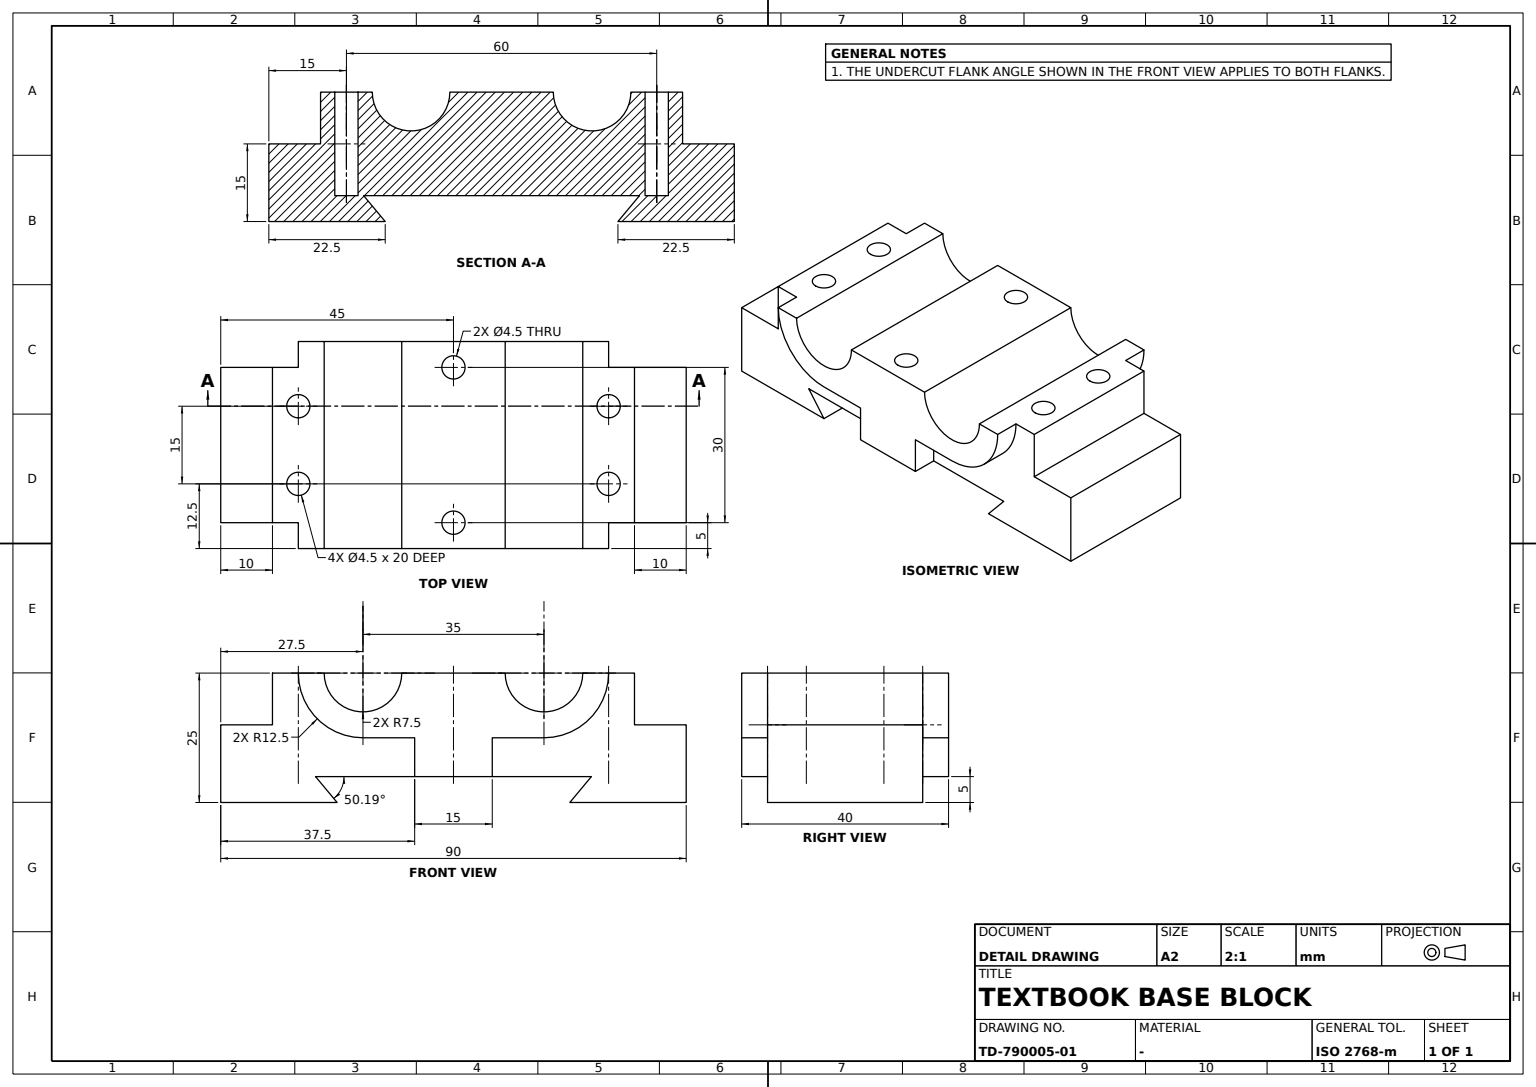
CATIA V5 part; units mm, degrees
sketch "Sketch1" plane through (0, 0, 0) normal (1, 0, 0) x (0, 1, 0)
  point P0 (-45, -5)
  line L0 (-45, -5) -> (-45, 10)
  point P1 (-45, 10)
  line L1 (-45, 10) -> (-35, 10)
  point P2 (-35, 10)
  line L2 (-35, 10) -> (-35, 20)
  point P3 (-35, 20)
  arc A0 (-25, 20) -> (-10, 20) centre (-17.5, 20) ccw
  line L3 (-35, 20) -> (-25, 20)
  point P4 (-30, 20)
  point P5 (-5, 20)
  point P6 (-10, 20)
  point P7 (-25, 20)
  line L4 (-10, 20) -> (-5, 20)
  line L5 (-45, -5) -> (-22.5, -5)
  point P8 (-22.5, -5)
  line L6 (-22.5, -5) -> (-26.6667, 0)
  point P9 (-26.6667, 0)
  point P10 (45, -5)
  point P11 (45, 10)
  point P12 (35, 10)
  point P13 (35, 20)
  point P14 (5, 20)
  point P15 (10, 20)
  point P16 (25, 20)
  point P17 (22.5, -5)
  point P18 (26.6667, 0)
  line L7 (45, -5) -> (45, 10)
  line L8 (45, 10) -> (35, 10)
  line L9 (35, 10) -> (35, 20)
  arc A1 (25, 20) -> (10, 20) centre (17.5, 20) cw
  line L10 (35, 20) -> (25, 20)
  line L11 (10, 20) -> (5, 20)
  line L12 (45, -5) -> (22.5, -5)
  line L13 (22.5, -5) -> (26.6667, 0)
  line L14 (-26.6667, 0) -> (26.6667, 0)
  point P19 (-17.5, 7.5)
  point P20 (-7.5, 0)
  line L15 (-5, 20) -> (5, 20)
  dimension "distance L1 P3" = 10
  dimension "distance P0 P1" = 15
  dimension "radius A0" = 7.5
  dimension "distance L0 P8" = 22.5
  dimension "distance L2 P1" = 10
  dimension "distance P9 L5" = 5
  dimension "distance P8 P17" = 45
  constraint vertical L0 y-axis
  constraint vertical L2 y-axis
  constraint horizontal L1 x-axis
  constraint horizontal L3 x-axis
  constraint horizontal L4 x-axis
  constraint horizontal L5 x-axis
  constraint horizontal L14 x-axis
  constraint horizontal L15 x-axis
  constraint coincidence L3 P4
  constraint coincidence L3 P5
  constraint coincidence L3 P6
  constraint coincidence L3 L4
  constraint coincidence L6 P2
  constraint coincidence L14 P20
  constraint symmetry P0 P10 y-axis
  constraint symmetry P1 P11 y-axis
  constraint symmetry P2 P12 y-axis
  constraint symmetry P3 P13 y-axis
  constraint symmetry P5 P14 y-axis
  constraint symmetry P6 P15 y-axis
  constraint symmetry P7 P16 y-axis
  constraint symmetry P8 P17 y-axis
  constraint symmetry P9 P18 y-axis
  constraint symmetry L0 L7 y-axis
  constraint symmetry L1 L8 y-axis
  constraint symmetry L2 L9 y-axis
  constraint symmetry A0 A1 y-axis
  constraint symmetry L3 L10 y-axis
  constraint symmetry L4 L11 y-axis
  constraint symmetry L5 L12 y-axis
  constraint symmetry L6 L13 y-axis
  constraint midpoint origin L14
extrude "Pad1" add sketch "Sketch1" along normal mid plane 30
sketch "Sketch2" plane through (15, 0, 0) normal (1, 0, 0) x (0, 1, 0)
  arc A0 (10, 20) -> (25, 20) centre (17.5, 20) ccw
  point P0 (10, 20)
  point P1 (25, 20)
  arc A1 (17.5, 7.5) -> (30, 20) centre (17.5, 20) ccw
  point P2 (17.5, 7.5)
  line L0 (17.5, 7.5) -> (7.5, 7.5)
  line L1 (35, 20) -> (25, 20) construction
  line L2 (30, 20) -> (25, 20)
  point P3 (35, 20)
  point P4 (25, 20)
  point P5 (30, 20)
  point P6 (7.5, 7.5)
  line L3 (-26.6667, 0) -> (26.6667, 0) construction
  line L4 (-7.5, 0) -> (7.5, 0)
  line L5 (7.5, 7.5) -> (7.5, 0)
  point P7 (7.5, 0)
  line L6 (5, 20) -> (-5, 20)
  line L7 (10, 20) -> (5, 20)
  line L8 (-5, 20) -> (-10, 20)
  point P8 (-10, 20)
  point P9 (-25, 20)
  point P10 (-10, 20)
  point P11 (-25, 20)
  point P12 (-35, 20)
  point P13 (-30, 20)
  point P14 (-17.5, 7.5)
  arc A2 (-17.5, 7.5) -> (-30, 20) centre (-17.5, 20) cw
  point P15 (-7.5, 7.5)
  line L9 (-17.5, 7.5) -> (-7.5, 7.5)
  point P16 (-7.5, 0)
  line L10 (-7.5, 7.5) -> (-7.5, 0)
  arc A3 (-10, 20) -> (-25, 20) centre (-17.5, 20) cw
  line L11 (-35, 20) -> (-25, 20) construction
  line L12 (-30, 20) -> (-25, 20)
  dimension "radius A1" = 12.5
  constraint concentricity A1 A0
  constraint tangency L0 A1
  constraint coincidence L1 P5
  constraint coincidence L3 P7
  constraint coincidence P1 P4
  constraint coincidence P8 P10
  constraint coincidence P9 P11
  constraint vertical L5 y-axis
  constraint symmetry P1 P9 y-axis
  constraint symmetry P0 P10 y-axis
  constraint symmetry A0 A3 y-axis
  constraint symmetry P4 P11 y-axis
  constraint symmetry P3 P12 y-axis
  constraint symmetry P5 P13 y-axis
  constraint symmetry L1 L11 y-axis
  constraint symmetry P2 P14 y-axis
  constraint symmetry A1 A2 y-axis
  constraint symmetry P6 P15 y-axis
  constraint symmetry L0 L9 y-axis
  constraint symmetry P7 P16 y-axis
  constraint symmetry L5 L10 y-axis
  constraint symmetry L1 L12 y-axis
extrude "Pad2" add sketch "Sketch2" along normal blind 5
mirror "Mirror1" about plane through (0, 0, 0) normal (1, 0, 0) of "Pad2"
sketch "Sketch3" plane through (0, 0, 0) normal (0, 0, 1) x (1, 0, 0)
  circle A0 centre (15, 0) radius 2.25
  point P0 (15, 0)
  circle A1 centre (7.5, 30) radius 2.25
  point P1 (7.5, 30)
  line L0 (-15, 35) -> (15, 35) construction
  line L1 (15, 35) -> (15, 25) construction
  circle A2 centre (-15, 0) radius 2.25
  circle A3 centre (-7.5, 30) radius 2.25
  circle A4 centre (-7.5, -30) radius 2.25
  circle A5 centre (7.5, -30) radius 2.25
  dimension "radius A0" = 2.25
  dimension "distance P0 y axis" = 15
  dimension "radius A1" = 2.25
  dimension "distance P1 L0" = 5
  dimension "distance P1 L1" = 7.5
  constraint coincidence P0 x-axis
  constraint symmetry A0 A2 y-axis
  constraint symmetry A1 A3 y-axis
  constraint symmetry A3 A4 x-axis
  constraint symmetry A1 A5 x-axis
extrude "Pocket1" cut sketch "Sketch3" along normal up to next
properties part number "base part"
